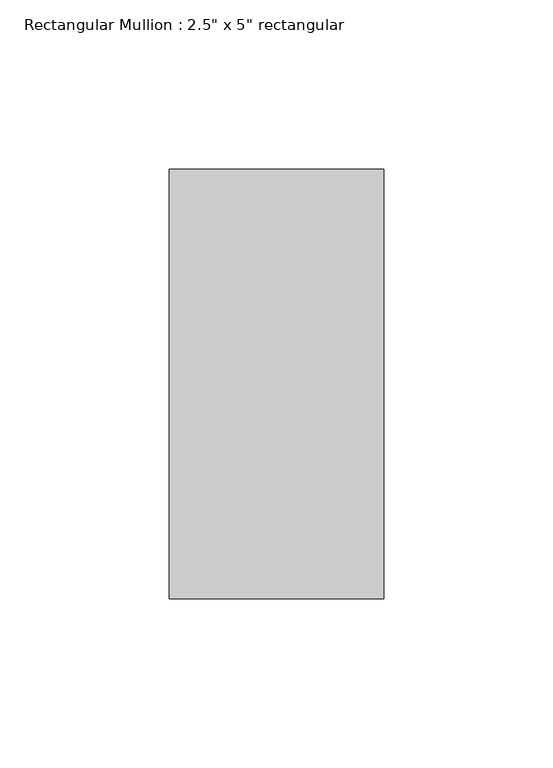
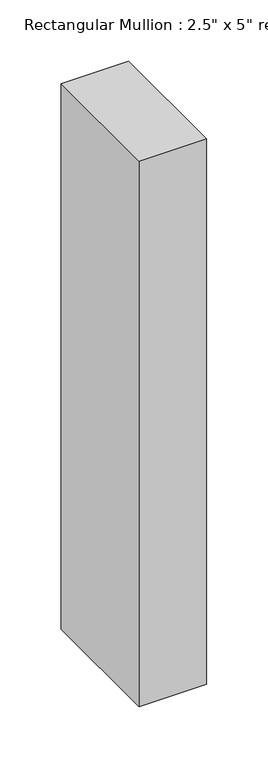
"""IFC4 building model written with IfcOpenShell, lengths in millimetres: member geometry."""

from ifc_helpers import new_model, si_unit, frame, origin, place, context, project, spatial, polyline, outline, extrude, source, transform, mapped, element, save


def member_b3e0441e(model_context):
    return source(origin(), model_context, "Body", "SweptSolid", [
        extrude(outline(polyline([(0.0, 63.5), (0.0, -63.5), (-63.5, -63.5), (-63.5, 63.5), (0.0, 63.5)])), frame((0.0, 0.0, -542.1748327), z_axis=(0.0, 0.0, 1.0), x_axis=(1.0, 0.0, 0.0)), (0.0, 0.0, 1.0), 542.1748327),
    ])


if __name__ == "__main__":
    model = new_model("IFC4")
    model_context = context("Model", 3, world=origin())
    ifc_project = project(units=[si_unit("LENGTHUNIT", "METRE", prefix="MILLI")], contexts=[model_context])
    site = spatial("IfcSite", under=ifc_project)
    building = spatial("IfcBuilding", under=site)
    placement = place(None, origin())
    member_shape = member_b3e0441e(model_context)
    element("IfcMember", 1, ObjectType="Rectangular Mullion : 2.5\" x 5\" rectangular", at=placement, inside=building, context=model_context, shape_type="MappedRepresentation", body=[
        mapped(member_shape, transform((0.0, 0.0, 0.0), x_axis=(1.0, 0.0, 0.0), y_axis=(0.0, 1.0, 0.0), z_axis=(0.0, 0.0, 1.0))),
    ])
    save(model, "model.ifc")

# Revit data of these elements
# Type "Rectangular Mullion : 2.5\" x 5\" rectangular"
#   built-in parameter 1007304 = 0.416667 (stored number, unit not read)
#   built-in parameter 1007301 = 0.104167 (stored number, unit not read)
#   built-in parameter 1007300 = 0.104167 (stored number, unit not read)
# Element 1 (IfcMember, "Rectangular Mullion : 2.5\" x 5\" rectangular")
#   Materials on its faces: "Aluminum"
# Materials
#   "Aluminum": class "Metal", colour RGB 247 247 247, transparency 0, Description = "Aluminum 6061", Cost = 0
